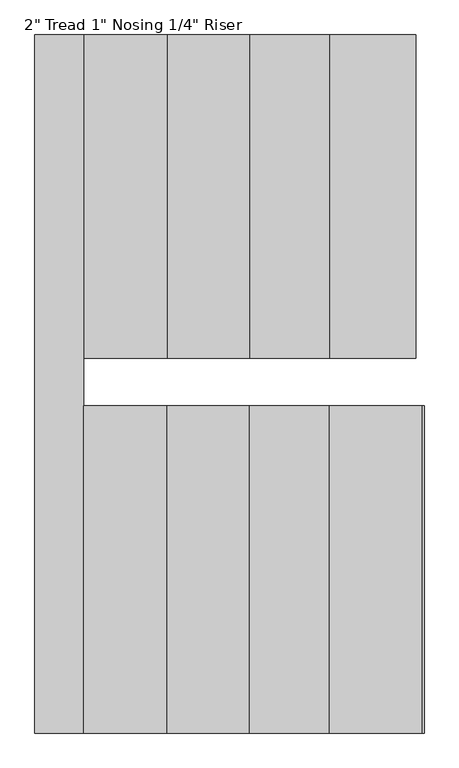
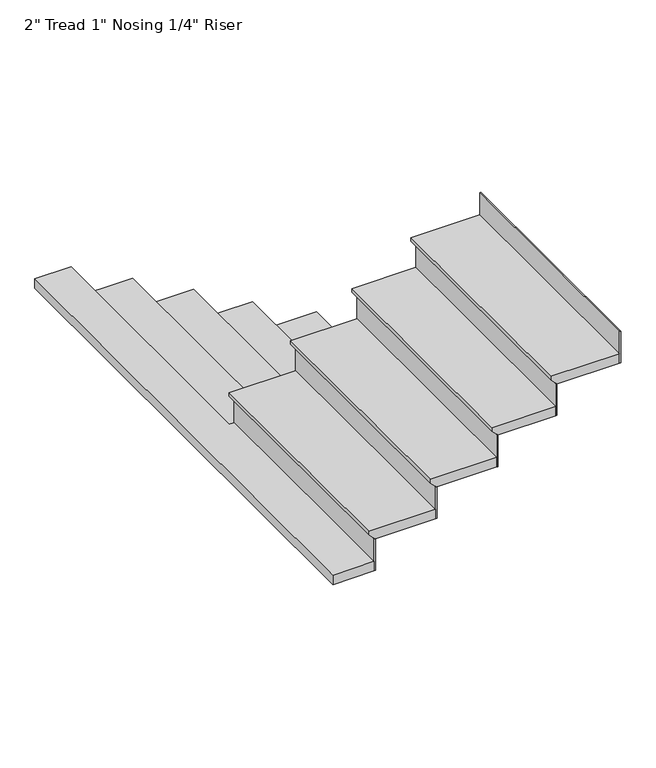
"""IFC4 building model written with IfcOpenShell, lengths in millimetres: stair flight geometry."""

from ifc_helpers import new_model, si_unit, origin, place, context, project, spatial, faceted_brep, source, transform, mapped, element, save


def stair_flight_e4a46180(model_context):
    return source(origin(), model_context, "Body", "Brep", [
        faceted_brep([(7105.1820958, 5486.4, 150.2833333), (7105.1820958, 5486.4, 169.3333333), (7105.1820958, 4274.6882626, 169.3333333), (7105.1820958, 4274.6882626, 150.2833333), (7079.7820958, 5486.4, 124.8833333), (7079.7820958, 4274.6882626, 124.8833333), (6756.4, 5486.4, 169.3333333), (6756.4, 4274.6882626, 169.3333333), (7079.7820958, 4274.6882626, 118.5333333), (6756.4, 4274.6882626, 118.5333333), (6756.4, 5486.4, 118.5333333), (7079.7820958, 5486.4, 118.5333333)], [[[0, 1, 2, 3]], [[4, 0, 3, 5]], [[2, 1, 6, 7]], [[8, 9, 10, 11]], [[2, 7, 9, 8, 5, 3]], [[8, 11, 4, 5]], [[6, 1, 0, 4, 11, 10]], [[7, 6, 10, 9]]]),
        faceted_brep([(7079.7820958, 5486.4, 118.5333333), (7079.7820958, 5486.4, 0.0), (7073.4320958, 5486.4, 0.0), (7073.4320958, 5486.4, 118.5333333), (7079.7820958, 4274.6882626, 118.5333333), (7073.4320958, 4274.6882626, 118.5333333), (7073.4320958, 4274.6882626, 0.0), (7079.7820958, 4274.6882626, 0.0)], [[[0, 1, 2, 3]], [[4, 5, 6, 7]], [[1, 0, 4, 7]], [[2, 1, 7, 6]], [[3, 2, 6, 5]], [[0, 3, 5, 4]]]),
        faceted_brep([(6756.4, 5486.4, 287.8666667), (6756.4, 5486.4, 118.5333333), (6750.05, 5486.4, 118.5333333), (6750.05, 5486.4, 287.8666667), (6756.4, 4274.6882626, 287.8666667), (6750.05, 4274.6882626, 287.8666667), (6750.05, 4274.6882626, 118.5333333), (6756.4, 4274.6882626, 118.5333333)], [[[0, 1, 2, 3]], [[4, 5, 6, 7]], [[1, 0, 4, 7]], [[2, 1, 7, 6]], [[3, 2, 6, 5]], [[0, 3, 5, 4]]]),
        faceted_brep([(6781.8, 4274.6882626, 338.6666667), (6781.8, 5486.4, 338.6666667), (6457.4820958, 5486.4, 338.6666667), (6457.4820958, 4274.6882626, 338.6666667), (6756.4, 4274.6882626, 287.8666667), (6457.4820958, 4274.6882626, 287.8666667), (6457.4820958, 5486.4, 287.8666667), (6756.4, 5486.4, 287.8666667), (6756.4, 4274.6882626, 294.2166667), (6781.8, 4274.6882626, 319.6166667), (6756.4, 5486.4, 294.2166667), (6781.8, 5486.4, 319.6166667)], [[[0, 1, 2, 3]], [[4, 5, 6, 7]], [[0, 3, 5, 4, 8, 9]], [[4, 7, 10, 8]], [[2, 1, 11, 10, 7, 6]], [[3, 2, 6, 5]], [[11, 1, 0, 9]], [[10, 11, 9, 8]]]),
        faceted_brep([(6457.4820958, 5486.4, 457.2), (6457.4820958, 5486.4, 287.8666667), (6451.1320958, 5486.4, 287.8666667), (6451.1320958, 5486.4, 457.2), (6457.4820958, 4274.6882626, 457.2), (6451.1320958, 4274.6882626, 457.2), (6451.1320958, 4274.6882626, 287.8666667), (6457.4820958, 4274.6882626, 287.8666667)], [[[0, 1, 2, 3]], [[4, 5, 6, 7]], [[1, 0, 4, 7]], [[2, 1, 7, 6]], [[3, 2, 6, 5]], [[0, 3, 5, 4]]]),
        faceted_brep([(6482.8820958, 4274.6882626, 508.0), (6482.8820958, 5486.4, 508.0), (6146.8, 5486.4, 508.0), (6146.8, 4274.6882626, 508.0), (6457.4820958, 4274.6882626, 457.2), (6146.8, 4274.6882626, 457.2), (6146.8, 5486.4, 457.2), (6457.4820958, 5486.4, 457.2), (6457.4820958, 4274.6882626, 463.55), (6482.8820958, 4274.6882626, 488.95), (6457.4820958, 5486.4, 463.55), (6482.8820958, 5486.4, 488.95)], [[[0, 1, 2, 3]], [[4, 5, 6, 7]], [[0, 3, 5, 4, 8, 9]], [[4, 7, 10, 8]], [[2, 1, 11, 10, 7, 6]], [[3, 2, 6, 5]], [[11, 1, 0, 9]], [[10, 11, 9, 8]]]),
        faceted_brep([(6146.8, 5486.4, 626.5333333), (6146.8, 5486.4, 457.2), (6140.45, 5486.4, 457.2), (6140.45, 5486.4, 626.5333333), (6146.8, 4274.6882626, 626.5333333), (6140.45, 4274.6882626, 626.5333333), (6140.45, 4274.6882626, 457.2), (6146.8, 4274.6882626, 457.2)], [[[0, 1, 2, 3]], [[4, 5, 6, 7]], [[1, 0, 4, 7]], [[2, 1, 7, 6]], [[3, 2, 6, 5]], [[0, 3, 5, 4]]]),
        faceted_brep([(6172.2, 4274.6882626, 677.3333333), (6172.2, 5486.4, 677.3333333), (5835.1820958, 5486.4, 677.3333333), (5835.1820958, 4274.6882626, 677.3333333), (6146.8, 4274.6882626, 626.5333333), (5835.1820958, 4274.6882626, 626.5333333), (5835.1820958, 5486.4, 626.5333333), (6146.8, 5486.4, 626.5333333), (6146.8, 4274.6882626, 632.8833333), (6172.2, 4274.6882626, 658.2833333), (6146.8, 5486.4, 632.8833333), (6172.2, 5486.4, 658.2833333)], [[[0, 1, 2, 3]], [[4, 5, 6, 7]], [[0, 3, 5, 4, 8, 9]], [[4, 7, 10, 8]], [[2, 1, 11, 10, 7, 6]], [[3, 2, 6, 5]], [[11, 1, 0, 9]], [[10, 11, 9, 8]]]),
        faceted_brep([(5835.1820958, 5486.4, 795.8666667), (5835.1820958, 5486.4, 626.5333333), (5828.8320958, 5486.4, 626.5333333), (5828.8320958, 5486.4, 795.8666667), (5835.1820958, 4274.6882626, 795.8666667), (5828.8320958, 4274.6882626, 795.8666667), (5828.8320958, 4274.6882626, 626.5333333), (5835.1820958, 4274.6882626, 626.5333333)], [[[0, 1, 2, 3]], [[4, 5, 6, 7]], [[1, 0, 4, 7]], [[2, 1, 7, 6]], [[3, 2, 6, 5]], [[0, 3, 5, 4]]]),
        faceted_brep([(5885.9820958, 4096.8882626, 846.6666667), (5860.5820958, 4096.8882626, 846.6666667), (5860.5820958, 5486.4, 846.6666667), (5676.9, 5486.4, 846.6666667), (5676.9, 2870.2, 846.6666667), (5885.9820958, 2870.2, 846.6666667), (5860.5820958, 4096.8882626, 795.8666667), (5885.9820958, 4096.8882626, 795.8666667), (5885.9820958, 2870.2, 795.8666667), (5676.9, 2870.2, 795.8666667), (5676.9, 5486.4, 795.8666667), (5835.1820958, 5486.4, 795.8666667), (5835.1820958, 4274.6882626, 795.8666667), (5860.5820958, 4274.6882626, 795.8666667), (5860.5820958, 4274.6882626, 827.6166667), (5860.5820958, 5486.4, 827.6166667), (5835.1820958, 4274.6882626, 802.2166667), (5835.1820958, 5486.4, 802.2166667)], [[[0, 1, 2, 3, 4, 5]], [[6, 7, 8, 9, 10, 11, 12, 13]], [[1, 0, 7, 6]], [[2, 1, 6, 13, 14, 15]], [[13, 12, 16, 14]], [[12, 11, 17, 16]], [[3, 2, 15, 17, 11, 10]], [[4, 3, 10, 9]], [[5, 4, 9, 8]], [[0, 5, 8, 7]], [[17, 15, 14, 16]]]),
        faceted_brep([(5885.9820958, 2870.2, 965.2), (5885.9820958, 2870.2, 795.8666667), (5892.3320958, 2870.2, 795.8666667), (5892.3320958, 2870.2, 965.2), (5885.9820958, 4096.8882626, 965.2), (5892.3320958, 4096.8882626, 965.2), (5892.3320958, 4096.8882626, 795.8666667), (5885.9820958, 4096.8882626, 795.8666667)], [[[0, 1, 2, 3]], [[4, 5, 6, 7]], [[1, 0, 4, 7]], [[2, 1, 7, 6]], [[3, 2, 6, 5]], [[0, 3, 5, 4]]]),
        faceted_brep([(5860.5820958, 4096.8882626, 1016.0), (5860.5820958, 2870.2, 1016.0), (6197.6, 2870.2, 1016.0), (6197.6, 4096.8882626, 1016.0), (5885.9820958, 4096.8882626, 965.2), (6197.6, 4096.8882626, 965.2), (6197.6, 2870.2, 965.2), (5885.9820958, 2870.2, 965.2), (5885.9820958, 4096.8882626, 971.55), (5860.5820958, 4096.8882626, 996.95), (5885.9820958, 2870.2, 971.55), (5860.5820958, 2870.2, 996.95)], [[[0, 1, 2, 3]], [[4, 5, 6, 7]], [[0, 3, 5, 4, 8, 9]], [[4, 7, 10, 8]], [[2, 1, 11, 10, 7, 6]], [[3, 2, 6, 5]], [[11, 1, 0, 9]], [[10, 11, 9, 8]]]),
        faceted_brep([(6197.6, 2870.2, 1134.5333333), (6197.6, 2870.2, 965.2), (6203.95, 2870.2, 965.2), (6203.95, 2870.2, 1134.5333333), (6197.6, 4096.8882626, 1134.5333333), (6203.95, 4096.8882626, 1134.5333333), (6203.95, 4096.8882626, 965.2), (6197.6, 4096.8882626, 965.2)], [[[0, 1, 2, 3]], [[4, 5, 6, 7]], [[1, 0, 4, 7]], [[2, 1, 7, 6]], [[3, 2, 6, 5]], [[0, 3, 5, 4]]]),
        faceted_brep([(6172.2, 4096.8882626, 1185.3333333), (6172.2, 2870.2, 1185.3333333), (6508.2820958, 2870.2, 1185.3333333), (6508.2820958, 4096.8882626, 1185.3333333), (6197.6, 4096.8882626, 1134.5333333), (6508.2820958, 4096.8882626, 1134.5333333), (6508.2820958, 2870.2, 1134.5333333), (6197.6, 2870.2, 1134.5333333), (6197.6, 4096.8882626, 1140.8833333), (6172.2, 4096.8882626, 1166.2833333), (6197.6, 2870.2, 1140.8833333), (6172.2, 2870.2, 1166.2833333)], [[[0, 1, 2, 3]], [[4, 5, 6, 7]], [[0, 3, 5, 4, 8, 9]], [[4, 7, 10, 8]], [[2, 1, 11, 10, 7, 6]], [[3, 2, 6, 5]], [[11, 1, 0, 9]], [[10, 11, 9, 8]]]),
        faceted_brep([(6508.2820958, 2870.2, 1303.8666667), (6508.2820958, 2870.2, 1134.5333333), (6514.6320958, 2870.2, 1134.5333333), (6514.6320958, 2870.2, 1303.8666667), (6508.2820958, 4096.8882626, 1303.8666667), (6514.6320958, 4096.8882626, 1303.8666667), (6514.6320958, 4096.8882626, 1134.5333333), (6508.2820958, 4096.8882626, 1134.5333333)], [[[0, 1, 2, 3]], [[4, 5, 6, 7]], [[1, 0, 4, 7]], [[2, 1, 7, 6]], [[3, 2, 6, 5]], [[0, 3, 5, 4]]]),
        faceted_brep([(6482.8820958, 4096.8882626, 1354.6666667), (6482.8820958, 2870.2, 1354.6666667), (6807.2, 2870.2, 1354.6666667), (6807.2, 4096.8882626, 1354.6666667), (6508.2820958, 4096.8882626, 1303.8666667), (6807.2, 4096.8882626, 1303.8666667), (6807.2, 2870.2, 1303.8666667), (6508.2820958, 2870.2, 1303.8666667), (6508.2820958, 4096.8882626, 1310.2166667), (6482.8820958, 4096.8882626, 1335.6166667), (6508.2820958, 2870.2, 1310.2166667), (6482.8820958, 2870.2, 1335.6166667)], [[[0, 1, 2, 3]], [[4, 5, 6, 7]], [[0, 3, 5, 4, 8, 9]], [[4, 7, 10, 8]], [[2, 1, 11, 10, 7, 6]], [[3, 2, 6, 5]], [[11, 1, 0, 9]], [[10, 11, 9, 8]]]),
        faceted_brep([(6807.2, 2870.2, 1473.2), (6807.2, 2870.2, 1303.8666667), (6813.55, 2870.2, 1303.8666667), (6813.55, 2870.2, 1473.2), (6807.2, 4096.8882626, 1473.2), (6813.55, 4096.8882626, 1473.2), (6813.55, 4096.8882626, 1303.8666667), (6807.2, 4096.8882626, 1303.8666667)], [[[0, 1, 2, 3]], [[4, 5, 6, 7]], [[1, 0, 4, 7]], [[2, 1, 7, 6]], [[3, 2, 6, 5]], [[0, 3, 5, 4]]]),
        faceted_brep([(7130.5820958, 2870.2, 1642.5333333), (7130.5820958, 2870.2, 1473.2), (7136.9320958, 2870.2, 1473.2), (7136.9320958, 2870.2, 1642.5333333), (7130.5820958, 4096.8882626, 1642.5333333), (7136.9320958, 4096.8882626, 1642.5333333), (7136.9320958, 4096.8882626, 1473.2), (7130.5820958, 4096.8882626, 1473.2)], [[[0, 1, 2, 3]], [[4, 5, 6, 7]], [[1, 0, 4, 7]], [[2, 1, 7, 6]], [[3, 2, 6, 5]], [[0, 3, 5, 4]]]),
        faceted_brep([(6781.8, 4096.8882626, 1524.0), (6781.8, 2870.2, 1524.0), (7130.5820958, 2870.2, 1524.0), (7130.5820958, 4096.8882626, 1524.0), (6807.2, 4096.8882626, 1473.2), (7130.5820958, 4096.8882626, 1473.2), (7130.5820958, 2870.2, 1473.2), (6807.2, 2870.2, 1473.2), (6807.2, 4096.8882626, 1479.55), (6781.8, 4096.8882626, 1504.95), (6807.2, 2870.2, 1479.55), (6781.8, 2870.2, 1504.95)], [[[0, 1, 2, 3]], [[4, 5, 6, 7]], [[0, 3, 5, 4, 8, 9]], [[4, 7, 10, 8]], [[2, 1, 11, 10, 7, 6]], [[3, 2, 6, 5]], [[11, 1, 0, 9]], [[10, 11, 9, 8]]]),
    ])


if __name__ == "__main__":
    model = new_model("IFC4")
    model_context = context("Model", 3, world=origin())
    ifc_project = project(units=[si_unit("LENGTHUNIT", "METRE", prefix="MILLI")], contexts=[model_context])
    site = spatial("IfcSite", under=ifc_project)
    building = spatial("IfcBuilding", under=site)
    placement = place(None, origin())
    stair_flight_shape = stair_flight_e4a46180(model_context)
    element("IfcStairFlight", 1, ObjectType="2\" Tread 1\" Nosing 1/4\" Riser", at=placement, inside=building, context=model_context, shape_type="MappedRepresentation", body=[
        mapped(stair_flight_shape, transform((0.0, 0.0, 0.0), x_axis=(1.0, 0.0, 0.0), y_axis=(0.0, 1.0, 0.0), z_axis=(0.0, 0.0, 1.0))),
    ])
    save(model, "model.ifc")
